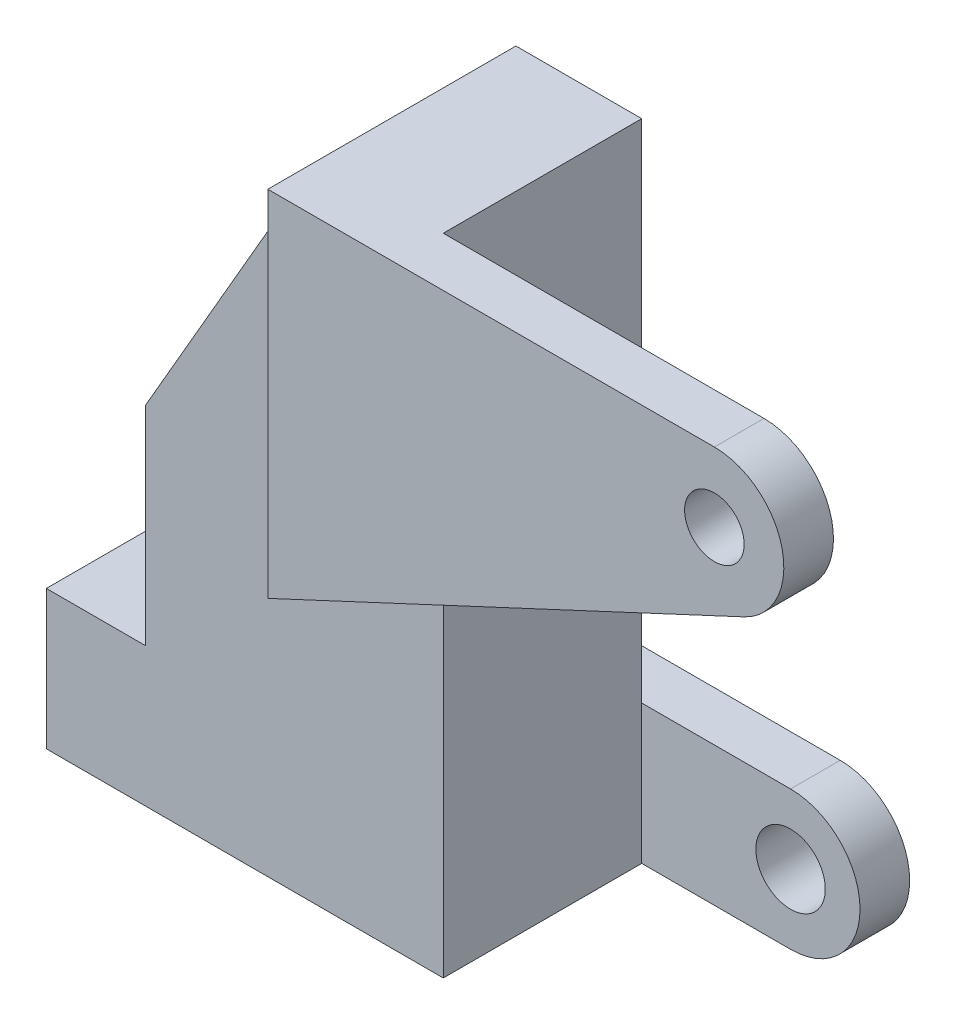
ISO-10303-21;
HEADER;
FILE_DESCRIPTION(('STEP AP214'),'2;1');
FILE_NAME('part.step','',(''),(''),'','','');
FILE_SCHEMA(('AUTOMOTIVE_DESIGN { 1 0 10303 214 1 1 1 1 }'));
ENDSEC;
DATA;
#1=APPLICATION_CONTEXT('core data for automotive mechanical design processes');
#2=APPLICATION_PROTOCOL_DEFINITION('international standard','automotive_design',2000,#1);
#3=PRODUCT_CONTEXT('',#1,'mechanical');
#4=PRODUCT('Part','Part','',(#3));
#5=PRODUCT_RELATED_PRODUCT_CATEGORY('part','',(#4));
#6=PRODUCT_DEFINITION_FORMATION('','',#4);
#7=PRODUCT_DEFINITION_CONTEXT('part definition',#1,'design');
#8=PRODUCT_DEFINITION('design','',#6,#7);
#9=PRODUCT_DEFINITION_SHAPE('','',#8);
#10=(LENGTH_UNIT() NAMED_UNIT(*) SI_UNIT(.MILLI.,.METRE.));
#11=(NAMED_UNIT(*) PLANE_ANGLE_UNIT() SI_UNIT($,.RADIAN.));
#12=(NAMED_UNIT(*) SI_UNIT($,.STERADIAN.) SOLID_ANGLE_UNIT());
#13=UNCERTAINTY_MEASURE_WITH_UNIT(LENGTH_MEASURE(1.E-05),#10,'distance_accuracy_value','');
#14=(GEOMETRIC_REPRESENTATION_CONTEXT(3) GLOBAL_UNCERTAINTY_ASSIGNED_CONTEXT((#13)) GLOBAL_UNIT_ASSIGNED_CONTEXT((#10,
#11,#12)) REPRESENTATION_CONTEXT('',''));
#15=CARTESIAN_POINT('',(0.,0.,0.));
#16=DIRECTION('',(0.,0.,1.));
#17=DIRECTION('',(1.,0.,0.));
#18=AXIS2_PLACEMENT_3D('',#15,#16,#17);
#19=CARTESIAN_POINT('',(0.,14.,0.));
#20=DIRECTION('',(0.,0.,1.));
#21=DIRECTION('',(1.,0.,0.));
#22=AXIS2_PLACEMENT_3D('',#19,#20,#21);
#23=PLANE('',#22);
#24=DIRECTION('',(0.,1.,0.));
#25=VECTOR('',#24,1.);
#26=CARTESIAN_POINT('',(10.,14.,0.));
#27=LINE('',#26,#25);
#28=CARTESIAN_POINT('',(10.,0.,0.));
#29=VERTEX_POINT('',#28);
#30=CARTESIAN_POINT('',(10.,14.,0.));
#31=VERTEX_POINT('',#30);
#32=EDGE_CURVE('E53',#29,#31,#27,.T.);
#33=ORIENTED_EDGE('',*,*,#32,.F.);
#34=DIRECTION('',(-1.,0.,0.));
#35=VECTOR('',#34,1.);
#36=CARTESIAN_POINT('',(0.,0.,0.));
#37=LINE('',#36,#35);
#38=CARTESIAN_POINT('',(0.,0.,0.));
#39=VERTEX_POINT('',#38);
#40=EDGE_CURVE('E245',#29,#39,#37,.T.);
#41=ORIENTED_EDGE('',*,*,#40,.T.);
#42=DIRECTION('',(0.,-1.,0.));
#43=VECTOR('',#42,1.);
#44=CARTESIAN_POINT('',(0.,14.,0.));
#45=LINE('',#44,#43);
#46=CARTESIAN_POINT('',(0.,14.,0.));
#47=VERTEX_POINT('',#46);
#48=EDGE_CURVE('E250',#47,#39,#45,.T.);
#49=ORIENTED_EDGE('',*,*,#48,.F.);
#50=DIRECTION('',(-1.,0.,0.));
#51=VECTOR('',#50,1.);
#52=CARTESIAN_POINT('',(0.,14.,0.));
#53=LINE('',#52,#51);
#54=EDGE_CURVE('E244',#31,#47,#53,.T.);
#55=ORIENTED_EDGE('',*,*,#54,.F.);
#56=EDGE_LOOP('',(#33,#41,#49,#55));
#57=FACE_BOUND('',#56,.T.);
#58=ADVANCED_FACE('F39',(#57),#23,.F.);
#59=DIRECTION('',(1.,0.,0.));
#60=VECTOR('',#59,1.);
#61=CARTESIAN_POINT('',(10.,14.,0.));
#62=LINE('',#61,#60);
#63=CARTESIAN_POINT('',(40.,14.,0.));
#64=VERTEX_POINT('',#63);
#65=EDGE_CURVE('E282',#31,#64,#62,.T.);
#66=ORIENTED_EDGE('',*,*,#65,.F.);
#67=DIRECTION('',(0.,-1.,0.));
#68=VECTOR('',#67,1.);
#69=CARTESIAN_POINT('',(10.,65.,0.));
#70=LINE('',#69,#68);
#71=CARTESIAN_POINT('',(10.,35.,0.));
#72=VERTEX_POINT('',#71);
#73=EDGE_CURVE('E234',#72,#31,#70,.T.);
#74=ORIENTED_EDGE('',*,*,#73,.F.);
#75=DIRECTION('',(0.499999999999995,0.866025403784442,0.));
#76=VECTOR('',#75,1.);
#77=CARTESIAN_POINT('',(-1.59326673973649,14.9198729810777,0.));
#78=LINE('',#77,#76);
#79=CARTESIAN_POINT('',(27.3205080756885,65.,0.));
#80=VERTEX_POINT('',#79);
#81=EDGE_CURVE('E219',#72,#80,#78,.T.);
#82=ORIENTED_EDGE('',*,*,#81,.T.);
#83=DIRECTION('',(-1.,0.,0.));
#84=VECTOR('',#83,1.);
#85=CARTESIAN_POINT('',(40.,65.,0.));
#86=LINE('',#85,#84);
#87=CARTESIAN_POINT('',(40.,65.,0.));
#88=VERTEX_POINT('',#87);
#89=EDGE_CURVE('E230',#88,#80,#86,.T.);
#90=ORIENTED_EDGE('',*,*,#89,.F.);
#91=DIRECTION('',(0.,-1.,0.));
#92=VECTOR('',#91,1.);
#93=CARTESIAN_POINT('',(40.,14.,0.));
#94=LINE('',#93,#92);
#95=EDGE_CURVE('E256',#88,#64,#94,.T.);
#96=ORIENTED_EDGE('',*,*,#95,.T.);
#97=EDGE_LOOP('',(#66,#74,#82,#90,#96));
#98=FACE_BOUND('',#97,.T.);
#99=ADVANCED_FACE('F319',(#98),#23,.F.);
#100=CARTESIAN_POINT('',(0.,14.,20.));
#101=DIRECTION('',(0.,0.,-1.));
#102=DIRECTION('',(-1.,0.,0.));
#103=AXIS2_PLACEMENT_3D('',#100,#101,#102);
#104=PLANE('',#103);
#105=DIRECTION('',(0.906307787036648,0.422618261740704,0.));
#106=VECTOR('',#105,1.);
#107=CARTESIAN_POINT('',(27.3205080756885,29.2925099502873,20.));
#108=LINE('',#107,#106);
#109=CARTESIAN_POINT('',(27.3205080756885,29.2925099502873,20.));
#110=VERTEX_POINT('',#109);
#111=CARTESIAN_POINT('',(40.,35.2050541361083,20.));
#112=VERTEX_POINT('',#111);
#113=EDGE_CURVE('E199',#110,#112,#108,.T.);
#114=ORIENTED_EDGE('',*,*,#113,.F.);
#115=DIRECTION('',(0.,-1.,0.));
#116=VECTOR('',#115,1.);
#117=CARTESIAN_POINT('',(27.3205080756885,65.,20.));
#118=LINE('',#117,#116);
#119=CARTESIAN_POINT('',(27.3205080756885,65.,20.));
#120=VERTEX_POINT('',#119);
#121=EDGE_CURVE('E198',#120,#110,#118,.T.);
#122=ORIENTED_EDGE('',*,*,#121,.F.);
#123=DIRECTION('',(0.499999999999995,0.866025403784442,0.));
#124=VECTOR('',#123,1.);
#125=CARTESIAN_POINT('',(10.,35.,20.));
#126=LINE('',#125,#124);
#127=CARTESIAN_POINT('',(10.,35.,20.));
#128=VERTEX_POINT('',#127);
#129=EDGE_CURVE('E214',#128,#120,#126,.T.);
#130=ORIENTED_EDGE('',*,*,#129,.F.);
#131=DIRECTION('',(0.,-1.,0.));
#132=VECTOR('',#131,1.);
#133=CARTESIAN_POINT('',(10.,65.,20.));
#134=LINE('',#133,#132);
#135=CARTESIAN_POINT('',(10.,14.,20.));
#136=VERTEX_POINT('',#135);
#137=EDGE_CURVE('E229',#128,#136,#134,.T.);
#138=ORIENTED_EDGE('',*,*,#137,.T.);
#139=DIRECTION('',(1.,0.,0.));
#140=VECTOR('',#139,1.);
#141=CARTESIAN_POINT('',(0.,14.,20.));
#142=LINE('',#141,#140);
#143=CARTESIAN_POINT('',(0.,14.,20.));
#144=VERTEX_POINT('',#143);
#145=EDGE_CURVE('E243',#144,#136,#142,.T.);
#146=ORIENTED_EDGE('',*,*,#145,.F.);
#147=DIRECTION('',(0.,-1.,0.));
#148=VECTOR('',#147,1.);
#149=CARTESIAN_POINT('',(0.,14.,20.));
#150=LINE('',#149,#148);
#151=CARTESIAN_POINT('',(0.,0.,20.));
#152=VERTEX_POINT('',#151);
#153=EDGE_CURVE('E50',#144,#152,#150,.T.);
#154=ORIENTED_EDGE('',*,*,#153,.T.);
#155=DIRECTION('',(1.,0.,0.));
#156=VECTOR('',#155,1.);
#157=CARTESIAN_POINT('',(0.,0.,20.));
#158=LINE('',#157,#156);
#159=CARTESIAN_POINT('',(40.,0.,20.));
#160=VERTEX_POINT('',#159);
#161=EDGE_CURVE('E247',#152,#160,#158,.T.);
#162=ORIENTED_EDGE('',*,*,#161,.T.);
#163=DIRECTION('',(0.,-1.,0.));
#164=VECTOR('',#163,1.);
#165=CARTESIAN_POINT('',(40.,14.,20.));
#166=LINE('',#165,#164);
#167=EDGE_CURVE('E65',#112,#160,#166,.T.);
#168=ORIENTED_EDGE('',*,*,#167,.F.);
#169=EDGE_LOOP('',(#114,#122,#130,#138,#146,#154,#162,#168));
#170=FACE_BOUND('',#169,.T.);
#171=ADVANCED_FACE('F263',(#170),#104,.F.);
#172=CARTESIAN_POINT('',(0.,14.,0.));
#173=DIRECTION('',(1.,0.,0.));
#174=DIRECTION('',(0.,0.,-1.));
#175=AXIS2_PLACEMENT_3D('',#172,#173,#174);
#176=PLANE('',#175);
#177=DIRECTION('',(0.,0.,1.));
#178=VECTOR('',#177,1.);
#179=CARTESIAN_POINT('',(0.,0.,0.));
#180=LINE('',#179,#178);
#181=EDGE_CURVE('E240',#39,#152,#180,.T.);
#182=ORIENTED_EDGE('',*,*,#181,.T.);
#183=ORIENTED_EDGE('',*,*,#153,.F.);
#184=DIRECTION('',(0.,0.,1.));
#185=VECTOR('',#184,1.);
#186=CARTESIAN_POINT('',(0.,14.,0.));
#187=LINE('',#186,#185);
#188=EDGE_CURVE('E236',#47,#144,#187,.T.);
#189=ORIENTED_EDGE('',*,*,#188,.F.);
#190=ORIENTED_EDGE('',*,*,#48,.T.);
#191=EDGE_LOOP('',(#182,#183,#189,#190));
#192=FACE_BOUND('',#191,.T.);
#193=ADVANCED_FACE('F41',(#192),#176,.F.);
#194=CARTESIAN_POINT('',(40.,14.,0.));
#195=DIRECTION('',(-1.,0.,0.));
#196=DIRECTION('',(0.,0.,1.));
#197=AXIS2_PLACEMENT_3D('',#194,#195,#196);
#198=PLANE('',#197);
#199=DIRECTION('',(0.,0.,-1.));
#200=VECTOR('',#199,1.);
#201=CARTESIAN_POINT('',(40.,0.,0.));
#202=LINE('',#201,#200);
#203=CARTESIAN_POINT('',(40.,0.,0.));
#204=VERTEX_POINT('',#203);
#205=EDGE_CURVE('E252',#160,#204,#202,.T.);
#206=ORIENTED_EDGE('',*,*,#205,.T.);
#207=EDGE_CURVE('E260',#64,#204,#94,.T.);
#208=ORIENTED_EDGE('',*,*,#207,.F.);
#209=ORIENTED_EDGE('',*,*,#95,.F.);
#210=DIRECTION('',(0.,0.,-1.));
#211=VECTOR('',#210,1.);
#212=CARTESIAN_POINT('',(40.,65.,0.));
#213=LINE('',#212,#211);
#214=CARTESIAN_POINT('',(40.,65.,20.));
#215=VERTEX_POINT('',#214);
#216=EDGE_CURVE('E221',#215,#88,#213,.T.);
#217=ORIENTED_EDGE('',*,*,#216,.F.);
#218=EDGE_CURVE('E257',#215,#112,#166,.T.);
#219=ORIENTED_EDGE('',*,*,#218,.T.);
#220=ORIENTED_EDGE('',*,*,#167,.T.);
#221=EDGE_LOOP('',(#206,#208,#209,#217,#219,#220));
#222=FACE_BOUND('',#221,.T.);
#223=ADVANCED_FACE('F280',(#222),#198,.F.);
#224=CARTESIAN_POINT('',(0.,14.,0.));
#225=DIRECTION('',(0.,1.,0.));
#226=DIRECTION('',(0.,0.,1.));
#227=AXIS2_PLACEMENT_3D('',#224,#225,#226);
#228=PLANE('',#227);
#229=DIRECTION('',(0.,0.,1.));
#230=VECTOR('',#229,1.);
#231=CARTESIAN_POINT('',(10.,14.,0.));
#232=LINE('',#231,#230);
#233=EDGE_CURVE('E224',#31,#136,#232,.T.);
#234=ORIENTED_EDGE('',*,*,#233,.F.);
#235=ORIENTED_EDGE('',*,*,#54,.T.);
#236=ORIENTED_EDGE('',*,*,#188,.T.);
#237=ORIENTED_EDGE('',*,*,#145,.T.);
#238=EDGE_LOOP('',(#234,#235,#236,#237));
#239=FACE_BOUND('',#238,.T.);
#240=ADVANCED_FACE('F329',(#239),#228,.T.);
#241=CARTESIAN_POINT('',(0.,0.,0.));
#242=DIRECTION('',(0.,1.,0.));
#243=DIRECTION('',(0.,0.,1.));
#244=AXIS2_PLACEMENT_3D('',#241,#242,#243);
#245=PLANE('',#244);
#246=ORIENTED_EDGE('',*,*,#181,.F.);
#247=ORIENTED_EDGE('',*,*,#40,.F.);
#248=DIRECTION('',(0.,0.,1.));
#249=VECTOR('',#248,1.);
#250=CARTESIAN_POINT('',(10.,0.,-5.));
#251=LINE('',#250,#249);
#252=CARTESIAN_POINT('',(10.,0.,-5.));
#253=VERTEX_POINT('',#252);
#254=EDGE_CURVE('E291',#253,#29,#251,.T.);
#255=ORIENTED_EDGE('',*,*,#254,.F.);
#256=DIRECTION('',(-1.,0.,0.));
#257=VECTOR('',#256,1.);
#258=CARTESIAN_POINT('',(10.,0.,-5.));
#259=LINE('',#258,#257);
#260=CARTESIAN_POINT('',(55.,0.,-5.));
#261=VERTEX_POINT('',#260);
#262=EDGE_CURVE('E163',#261,#253,#259,.T.);
#263=ORIENTED_EDGE('',*,*,#262,.F.);
#264=DIRECTION('',(0.,0.,1.));
#265=VECTOR('',#264,1.);
#266=CARTESIAN_POINT('',(55.,0.,-5.));
#267=LINE('',#266,#265);
#268=CARTESIAN_POINT('',(55.,0.,0.));
#269=VERTEX_POINT('',#268);
#270=EDGE_CURVE('E178',#261,#269,#267,.T.);
#271=ORIENTED_EDGE('',*,*,#270,.T.);
#272=DIRECTION('',(-1.,0.,0.));
#273=VECTOR('',#272,1.);
#274=CARTESIAN_POINT('',(10.,0.,0.));
#275=LINE('',#274,#273);
#276=EDGE_CURVE('E169',#269,#204,#275,.T.);
#277=ORIENTED_EDGE('',*,*,#276,.T.);
#278=ORIENTED_EDGE('',*,*,#205,.F.);
#279=ORIENTED_EDGE('',*,*,#161,.F.);
#280=EDGE_LOOP('',(#246,#247,#255,#263,#271,#277,#278,#279));
#281=FACE_BOUND('',#280,.T.);
#282=ADVANCED_FACE('F269',(#281),#245,.F.);
#283=CARTESIAN_POINT('',(10.,65.,0.));
#284=DIRECTION('',(1.,0.,0.));
#285=DIRECTION('',(0.,0.,-1.));
#286=AXIS2_PLACEMENT_3D('',#283,#284,#285);
#287=PLANE('',#286);
#288=ORIENTED_EDGE('',*,*,#137,.F.);
#289=DIRECTION('',(0.,0.,1.));
#290=VECTOR('',#289,1.);
#291=CARTESIAN_POINT('',(10.,35.,-31.));
#292=LINE('',#291,#290);
#293=EDGE_CURVE('E217',#72,#128,#292,.T.);
#294=ORIENTED_EDGE('',*,*,#293,.F.);
#295=ORIENTED_EDGE('',*,*,#73,.T.);
#296=ORIENTED_EDGE('',*,*,#233,.T.);
#297=EDGE_LOOP('',(#288,#294,#295,#296));
#298=FACE_BOUND('',#297,.T.);
#299=ADVANCED_FACE('F364',(#298),#287,.F.);
#300=CARTESIAN_POINT('',(0.,65.,0.));
#301=DIRECTION('',(0.,-1.,0.));
#302=DIRECTION('',(0.,0.,-1.));
#303=AXIS2_PLACEMENT_3D('',#300,#301,#302);
#304=PLANE('',#303);
#305=ORIENTED_EDGE('',*,*,#89,.T.);
#306=DIRECTION('',(0.,0.,1.));
#307=VECTOR('',#306,1.);
#308=CARTESIAN_POINT('',(27.3205080756885,65.,0.));
#309=LINE('',#308,#307);
#310=EDGE_CURVE('E11',#80,#120,#309,.T.);
#311=ORIENTED_EDGE('',*,*,#310,.T.);
#312=DIRECTION('',(0.,0.,-1.));
#313=VECTOR('',#312,1.);
#314=CARTESIAN_POINT('',(27.3205080756885,65.,25.));
#315=LINE('',#314,#313);
#316=CARTESIAN_POINT('',(27.3205080756885,65.,25.));
#317=VERTEX_POINT('',#316);
#318=EDGE_CURVE('E215',#317,#120,#315,.T.);
#319=ORIENTED_EDGE('',*,*,#318,.F.);
#320=DIRECTION('',(-1.,0.,0.));
#321=VECTOR('',#320,1.);
#322=CARTESIAN_POINT('',(27.3205080756885,65.,25.));
#323=LINE('',#322,#321);
#324=CARTESIAN_POINT('',(72.3205080756885,65.,25.));
#325=VERTEX_POINT('',#324);
#326=EDGE_CURVE('E181',#325,#317,#323,.T.);
#327=ORIENTED_EDGE('',*,*,#326,.F.);
#328=DIRECTION('',(0.,0.,-1.));
#329=VECTOR('',#328,1.);
#330=CARTESIAN_POINT('',(72.3205080756885,65.,25.));
#331=LINE('',#330,#329);
#332=CARTESIAN_POINT('',(72.3205080756885,65.,20.));
#333=VERTEX_POINT('',#332);
#334=EDGE_CURVE('E191',#325,#333,#331,.T.);
#335=ORIENTED_EDGE('',*,*,#334,.T.);
#336=DIRECTION('',(-1.,0.,0.));
#337=VECTOR('',#336,1.);
#338=CARTESIAN_POINT('',(27.3205080756885,65.,20.));
#339=LINE('',#338,#337);
#340=EDGE_CURVE('E182',#333,#215,#339,.T.);
#341=ORIENTED_EDGE('',*,*,#340,.T.);
#342=ORIENTED_EDGE('',*,*,#216,.T.);
#343=EDGE_LOOP('',(#305,#311,#319,#327,#335,#341,#342));
#344=FACE_BOUND('',#343,.T.);
#345=ADVANCED_FACE('F442',(#344),#304,.F.);
#346=CARTESIAN_POINT('',(10.,35.,-31.));
#347=DIRECTION('',(0.866025403784442,-0.499999999999995,0.));
#348=DIRECTION('',(0.499999999999995,0.866025403784442,0.));
#349=AXIS2_PLACEMENT_3D('',#346,#347,#348);
#350=PLANE('',#349);
#351=ORIENTED_EDGE('',*,*,#293,.T.);
#352=ORIENTED_EDGE('',*,*,#129,.T.);
#353=ORIENTED_EDGE('',*,*,#310,.F.);
#354=ORIENTED_EDGE('',*,*,#81,.F.);
#355=EDGE_LOOP('',(#351,#352,#353,#354));
#356=FACE_BOUND('',#355,.T.);
#357=ADVANCED_FACE('F421',(#356),#350,.F.);
#358=CARTESIAN_POINT('',(72.3205080756885,58.,25.));
#359=DIRECTION('',(0.,0.,1.));
#360=DIRECTION('',(1.,0.,0.));
#361=AXIS2_PLACEMENT_3D('',#358,#359,#360);
#362=PLANE('',#361);
#363=ORIENTED_EDGE('',*,*,#326,.T.);
#364=DIRECTION('',(0.,-1.,0.));
#365=VECTOR('',#364,1.);
#366=CARTESIAN_POINT('',(27.3205080756885,65.,25.));
#367=LINE('',#366,#365);
#368=CARTESIAN_POINT('',(27.3205080756885,29.2925099502873,25.));
#369=VERTEX_POINT('',#368);
#370=EDGE_CURVE('E188',#317,#369,#367,.T.);
#371=ORIENTED_EDGE('',*,*,#370,.T.);
#372=DIRECTION('',(0.906307787036648,0.422618261740704,0.));
#373=VECTOR('',#372,1.);
#374=CARTESIAN_POINT('',(27.3205080756885,29.2925099502873,25.));
#375=LINE('',#374,#373);
#376=CARTESIAN_POINT('',(75.2788359078735,51.6558454907435,25.));
#377=VERTEX_POINT('',#376);
#378=EDGE_CURVE('E187',#369,#377,#375,.T.);
#379=ORIENTED_EDGE('',*,*,#378,.T.);
#380=CARTESIAN_POINT('',(72.3205080756885,58.,25.));
#381=DIRECTION('',(0.,0.,1.));
#382=DIRECTION('',(1.,0.,0.));
#383=AXIS2_PLACEMENT_3D('',#380,#381,#382);
#384=CIRCLE('',#383,6.99999999999999);
#385=EDGE_CURVE('E193',#377,#325,#384,.T.);
#386=ORIENTED_EDGE('',*,*,#385,.T.);
#387=EDGE_LOOP('',(#363,#371,#379,#386));
#388=FACE_BOUND('',#387,.T.);
#389=CARTESIAN_POINT('',(72.3205080756885,58.,25.));
#390=DIRECTION('',(0.,0.,1.));
#391=DIRECTION('',(1.,0.,0.));
#392=AXIS2_PLACEMENT_3D('',#389,#390,#391);
#393=CIRCLE('',#392,3.00000000000001);
#394=CARTESIAN_POINT('',(75.3205080756885,58.,25.));
#395=VERTEX_POINT('',#394);
#396=EDGE_CURVE('E172',#395,#395,#393,.T.);
#397=ORIENTED_EDGE('',*,*,#396,.F.);
#398=EDGE_LOOP('',(#397));
#399=FACE_BOUND('',#398,.T.);
#400=ADVANCED_FACE('F420',(#388,#399),#362,.T.);
#401=CARTESIAN_POINT('',(72.3205080756885,58.,20.));
#402=DIRECTION('',(0.,0.,1.));
#403=DIRECTION('',(1.,0.,0.));
#404=AXIS2_PLACEMENT_3D('',#401,#402,#403);
#405=PLANE('',#404);
#406=ORIENTED_EDGE('',*,*,#218,.F.);
#407=ORIENTED_EDGE('',*,*,#340,.F.);
#408=CARTESIAN_POINT('',(72.3205080756885,58.,20.));
#409=DIRECTION('',(0.,0.,1.));
#410=DIRECTION('',(1.,0.,0.));
#411=AXIS2_PLACEMENT_3D('',#408,#409,#410);
#412=CIRCLE('',#411,6.99999999999999);
#413=CARTESIAN_POINT('',(75.2788359078735,51.6558454907435,20.));
#414=VERTEX_POINT('',#413);
#415=EDGE_CURVE('E190',#414,#333,#412,.T.);
#416=ORIENTED_EDGE('',*,*,#415,.F.);
#417=EDGE_CURVE('E200',#112,#414,#108,.T.);
#418=ORIENTED_EDGE('',*,*,#417,.F.);
#419=EDGE_LOOP('',(#406,#407,#416,#418));
#420=FACE_BOUND('',#419,.T.);
#421=CARTESIAN_POINT('',(72.3205080756885,58.,20.));
#422=DIRECTION('',(0.,0.,1.));
#423=DIRECTION('',(1.,0.,0.));
#424=AXIS2_PLACEMENT_3D('',#421,#422,#423);
#425=CIRCLE('',#424,3.00000000000001);
#426=CARTESIAN_POINT('',(75.3205080756885,58.,20.));
#427=VERTEX_POINT('',#426);
#428=EDGE_CURVE('E173',#427,#427,#425,.T.);
#429=ORIENTED_EDGE('',*,*,#428,.T.);
#430=EDGE_LOOP('',(#429));
#431=FACE_BOUND('',#430,.T.);
#432=ADVANCED_FACE('F425',(#420,#431),#405,.F.);
#433=CARTESIAN_POINT('',(27.3205080756885,65.,25.));
#434=DIRECTION('',(1.,0.,0.));
#435=DIRECTION('',(0.,1.,0.));
#436=AXIS2_PLACEMENT_3D('',#433,#434,#435);
#437=PLANE('',#436);
#438=ORIENTED_EDGE('',*,*,#121,.T.);
#439=DIRECTION('',(0.,0.,-1.));
#440=VECTOR('',#439,1.);
#441=CARTESIAN_POINT('',(27.3205080756885,29.2925099502873,25.));
#442=LINE('',#441,#440);
#443=EDGE_CURVE('E207',#369,#110,#442,.T.);
#444=ORIENTED_EDGE('',*,*,#443,.F.);
#445=ORIENTED_EDGE('',*,*,#370,.F.);
#446=ORIENTED_EDGE('',*,*,#318,.T.);
#447=EDGE_LOOP('',(#438,#444,#445,#446));
#448=FACE_BOUND('',#447,.T.);
#449=ADVANCED_FACE('F430',(#448),#437,.F.);
#450=CARTESIAN_POINT('',(27.3205080756885,29.2925099502873,25.));
#451=DIRECTION('',(-0.422618261740704,0.906307787036648,0.));
#452=DIRECTION('',(-0.906307787036648,-0.422618261740704,0.));
#453=AXIS2_PLACEMENT_3D('',#450,#451,#452);
#454=PLANE('',#453);
#455=ORIENTED_EDGE('',*,*,#113,.T.);
#456=ORIENTED_EDGE('',*,*,#417,.T.);
#457=DIRECTION('',(0.,0.,-1.));
#458=VECTOR('',#457,1.);
#459=CARTESIAN_POINT('',(75.2788359078735,51.6558454907435,25.));
#460=LINE('',#459,#458);
#461=EDGE_CURVE('E206',#377,#414,#460,.T.);
#462=ORIENTED_EDGE('',*,*,#461,.F.);
#463=ORIENTED_EDGE('',*,*,#378,.F.);
#464=ORIENTED_EDGE('',*,*,#443,.T.);
#465=EDGE_LOOP('',(#455,#456,#462,#463,#464));
#466=FACE_BOUND('',#465,.T.);
#467=ADVANCED_FACE('F431',(#466),#454,.F.);
#468=CARTESIAN_POINT('',(72.3205080756885,58.,25.));
#469=DIRECTION('',(0.,0.,-1.));
#470=DIRECTION('',(-1.,0.,0.));
#471=AXIS2_PLACEMENT_3D('',#468,#469,#470);
#472=CYLINDRICAL_SURFACE('',#471,6.99999999999999);
#473=ORIENTED_EDGE('',*,*,#415,.T.);
#474=ORIENTED_EDGE('',*,*,#334,.F.);
#475=ORIENTED_EDGE('',*,*,#385,.F.);
#476=ORIENTED_EDGE('',*,*,#461,.T.);
#477=EDGE_LOOP('',(#473,#474,#475,#476));
#478=FACE_BOUND('',#477,.T.);
#479=ADVANCED_FACE('F417',(#478),#472,.T.);
#480=CARTESIAN_POINT('',(72.3205080756885,58.,25.));
#481=DIRECTION('',(0.,0.,-1.));
#482=DIRECTION('',(-1.,0.,0.));
#483=AXIS2_PLACEMENT_3D('',#480,#481,#482);
#484=CYLINDRICAL_SURFACE('',#483,3.00000000000001);
#485=ORIENTED_EDGE('',*,*,#396,.T.);
#486=EDGE_LOOP('',(#485));
#487=FACE_BOUND('',#486,.T.);
#488=ORIENTED_EDGE('',*,*,#428,.F.);
#489=EDGE_LOOP('',(#488));
#490=FACE_BOUND('',#489,.T.);
#491=ADVANCED_FACE('F312',(#487,#490),#484,.F.);
#492=CARTESIAN_POINT('',(55.,7.,0.));
#493=DIRECTION('',(0.,0.,-1.));
#494=DIRECTION('',(-1.,0.,0.));
#495=AXIS2_PLACEMENT_3D('',#492,#493,#494);
#496=PLANE('',#495);
#497=CARTESIAN_POINT('',(55.,7.,0.));
#498=DIRECTION('',(0.,0.,-1.));
#499=DIRECTION('',(-1.,0.,0.));
#500=AXIS2_PLACEMENT_3D('',#497,#498,#499);
#501=CIRCLE('',#500,3.5);
#502=CARTESIAN_POINT('',(51.5,7.,0.));
#503=VERTEX_POINT('',#502);
#504=EDGE_CURVE('E297',#503,#503,#501,.T.);
#505=ORIENTED_EDGE('',*,*,#504,.T.);
#506=EDGE_LOOP('',(#505));
#507=FACE_BOUND('',#506,.T.);
#508=CARTESIAN_POINT('',(55.,14.,0.));
#509=VERTEX_POINT('',#508);
#510=EDGE_CURVE('E285',#64,#509,#62,.T.);
#511=ORIENTED_EDGE('',*,*,#510,.F.);
#512=ORIENTED_EDGE('',*,*,#207,.T.);
#513=ORIENTED_EDGE('',*,*,#276,.F.);
#514=CARTESIAN_POINT('',(55.,7.,0.));
#515=DIRECTION('',(0.,0.,-1.));
#516=DIRECTION('',(-1.,0.,0.));
#517=AXIS2_PLACEMENT_3D('',#514,#515,#516);
#518=CIRCLE('',#517,7.);
#519=EDGE_CURVE('E281',#509,#269,#518,.T.);
#520=ORIENTED_EDGE('',*,*,#519,.F.);
#521=EDGE_LOOP('',(#511,#512,#513,#520));
#522=FACE_BOUND('',#521,.T.);
#523=ADVANCED_FACE('F278',(#507,#522),#496,.F.);
#524=CARTESIAN_POINT('',(55.,7.,-5.));
#525=DIRECTION('',(0.,0.,-1.));
#526=DIRECTION('',(-1.,0.,0.));
#527=AXIS2_PLACEMENT_3D('',#524,#525,#526);
#528=PLANE('',#527);
#529=DIRECTION('',(0.,1.,0.));
#530=VECTOR('',#529,1.);
#531=CARTESIAN_POINT('',(10.,14.,-5.));
#532=LINE('',#531,#530);
#533=CARTESIAN_POINT('',(10.,14.,-5.));
#534=VERTEX_POINT('',#533);
#535=EDGE_CURVE('E158',#253,#534,#532,.T.);
#536=ORIENTED_EDGE('',*,*,#535,.T.);
#537=DIRECTION('',(1.,0.,0.));
#538=VECTOR('',#537,1.);
#539=CARTESIAN_POINT('',(10.,14.,-5.));
#540=LINE('',#539,#538);
#541=CARTESIAN_POINT('',(55.,14.,-5.));
#542=VERTEX_POINT('',#541);
#543=EDGE_CURVE('E150',#534,#542,#540,.T.);
#544=ORIENTED_EDGE('',*,*,#543,.T.);
#545=CARTESIAN_POINT('',(55.,7.,-5.));
#546=DIRECTION('',(0.,0.,-1.));
#547=DIRECTION('',(-1.,0.,0.));
#548=AXIS2_PLACEMENT_3D('',#545,#546,#547);
#549=CIRCLE('',#548,7.);
#550=EDGE_CURVE('E160',#542,#261,#549,.T.);
#551=ORIENTED_EDGE('',*,*,#550,.T.);
#552=ORIENTED_EDGE('',*,*,#262,.T.);
#553=EDGE_LOOP('',(#536,#544,#551,#552));
#554=FACE_BOUND('',#553,.T.);
#555=CARTESIAN_POINT('',(55.,7.,-5.));
#556=DIRECTION('',(0.,0.,-1.));
#557=DIRECTION('',(-1.,0.,0.));
#558=AXIS2_PLACEMENT_3D('',#555,#556,#557);
#559=CIRCLE('',#558,3.5);
#560=CARTESIAN_POINT('',(51.5,7.,-5.));
#561=VERTEX_POINT('',#560);
#562=EDGE_CURVE('E305',#561,#561,#559,.T.);
#563=ORIENTED_EDGE('',*,*,#562,.F.);
#564=EDGE_LOOP('',(#563));
#565=FACE_BOUND('',#564,.T.);
#566=ADVANCED_FACE('F161',(#554,#565),#528,.T.);
#567=CARTESIAN_POINT('',(10.,14.,-5.));
#568=DIRECTION('',(1.,0.,0.));
#569=DIRECTION('',(0.,0.,-1.));
#570=AXIS2_PLACEMENT_3D('',#567,#568,#569);
#571=PLANE('',#570);
#572=ORIENTED_EDGE('',*,*,#32,.T.);
#573=DIRECTION('',(0.,0.,1.));
#574=VECTOR('',#573,1.);
#575=CARTESIAN_POINT('',(10.,14.,-5.));
#576=LINE('',#575,#574);
#577=EDGE_CURVE('E155',#534,#31,#576,.T.);
#578=ORIENTED_EDGE('',*,*,#577,.F.);
#579=ORIENTED_EDGE('',*,*,#535,.F.);
#580=ORIENTED_EDGE('',*,*,#254,.T.);
#581=EDGE_LOOP('',(#572,#578,#579,#580));
#582=FACE_BOUND('',#581,.T.);
#583=ADVANCED_FACE('F168',(#582),#571,.F.);
#584=CARTESIAN_POINT('',(10.,14.,-5.));
#585=DIRECTION('',(0.,-1.,0.));
#586=DIRECTION('',(1.,0.,0.));
#587=AXIS2_PLACEMENT_3D('',#584,#585,#586);
#588=PLANE('',#587);
#589=ORIENTED_EDGE('',*,*,#65,.T.);
#590=ORIENTED_EDGE('',*,*,#510,.T.);
#591=DIRECTION('',(0.,0.,1.));
#592=VECTOR('',#591,1.);
#593=CARTESIAN_POINT('',(55.,14.,-5.));
#594=LINE('',#593,#592);
#595=EDGE_CURVE('E152',#542,#509,#594,.T.);
#596=ORIENTED_EDGE('',*,*,#595,.F.);
#597=ORIENTED_EDGE('',*,*,#543,.F.);
#598=ORIENTED_EDGE('',*,*,#577,.T.);
#599=EDGE_LOOP('',(#589,#590,#596,#597,#598));
#600=FACE_BOUND('',#599,.T.);
#601=ADVANCED_FACE('F147',(#600),#588,.F.);
#602=CARTESIAN_POINT('',(55.,7.,-5.));
#603=DIRECTION('',(0.,0.,1.));
#604=DIRECTION('',(1.,0.,0.));
#605=AXIS2_PLACEMENT_3D('',#602,#603,#604);
#606=CYLINDRICAL_SURFACE('',#605,7.);
#607=ORIENTED_EDGE('',*,*,#519,.T.);
#608=ORIENTED_EDGE('',*,*,#270,.F.);
#609=ORIENTED_EDGE('',*,*,#550,.F.);
#610=ORIENTED_EDGE('',*,*,#595,.T.);
#611=EDGE_LOOP('',(#607,#608,#609,#610));
#612=FACE_BOUND('',#611,.T.);
#613=ADVANCED_FACE('F298',(#612),#606,.T.);
#614=CARTESIAN_POINT('',(55.,7.,-5.));
#615=DIRECTION('',(0.,0.,1.));
#616=DIRECTION('',(1.,0.,0.));
#617=AXIS2_PLACEMENT_3D('',#614,#615,#616);
#618=CYLINDRICAL_SURFACE('',#617,3.5);
#619=ORIENTED_EDGE('',*,*,#562,.T.);
#620=EDGE_LOOP('',(#619));
#621=FACE_BOUND('',#620,.T.);
#622=ORIENTED_EDGE('',*,*,#504,.F.);
#623=EDGE_LOOP('',(#622));
#624=FACE_BOUND('',#623,.T.);
#625=ADVANCED_FACE('F308',(#621,#624),#618,.F.);
#626=CLOSED_SHELL('',(#58,#99,#171,#193,#223,#240,#282,#299,#345,#357,#400,#432,#449,#467,#479,
#491,#523,#566,#583,#601,#613,#625));
#627=MANIFOLD_SOLID_BREP('B2',#626);
#628=ADVANCED_BREP_SHAPE_REPRESENTATION('',(#18,#627),#14);
#629=SHAPE_DEFINITION_REPRESENTATION(#9,#628);
ENDSEC;
END-ISO-10303-21;
